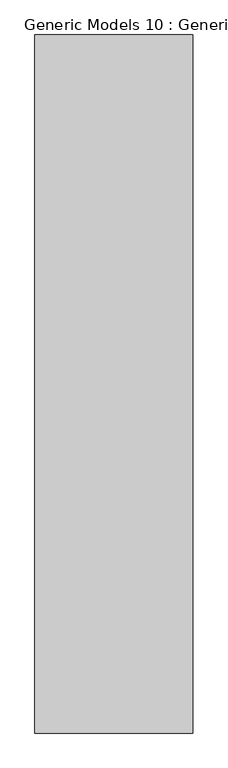
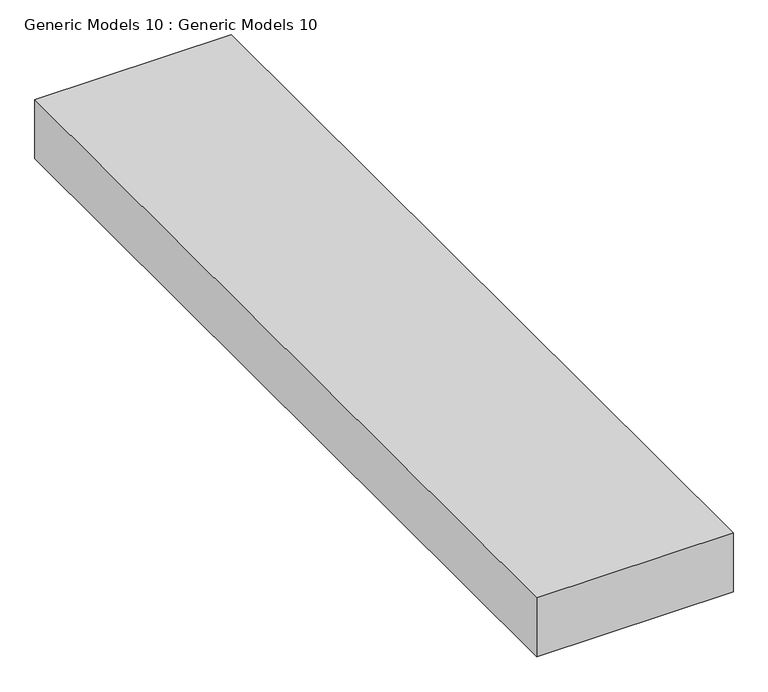
"""IFC4 building model written with IfcOpenShell, lengths in millimetres: proxy geometry, Generic Models 10 : Generic Models 10."""

from ifc_helpers import new_model, si_unit, frame, origin, place, context, project, spatial, polyline, outline, extrude, source, transform, mapped, element, save


def generic_models_10_generic_models_10_e59920a7(model_context):
    return source(origin(), model_context, "Body", "SweptSolid", [
        extrude(outline(polyline([(-3320.2262478, 2441.9722768), (-3320.2262478, 307.998934), (-3802.4859258, 307.998934), (-3802.4859258, 2441.9722768), (-3320.2262478, 2441.9722768)])), frame((0.0, 0.0, 5279.0460342), z_axis=(0.0, 0.0, 1.0), x_axis=(1.0, 0.0, 0.0)), (0.0, 0.0, 1.0), 152.4),
    ])


if __name__ == "__main__":
    model = new_model("IFC4")
    model_context = context("Model", 3, world=origin())
    ifc_project = project(units=[si_unit("LENGTHUNIT", "METRE", prefix="MILLI")], contexts=[model_context])
    site = spatial("IfcSite", under=ifc_project)
    building = spatial("IfcBuilding", under=site)
    placement = place(None, origin())
    generic_models_10_generic_models_10_shape = generic_models_10_generic_models_10_e59920a7(model_context)
    element("IfcBuildingElementProxy", 1, Name="Generic Models 10 : Generic Models 10", ObjectType="Generic Models 10 : Generic Models 10", at=placement, inside=building, context=model_context, shape_type="MappedRepresentation", body=[
        mapped(generic_models_10_generic_models_10_shape, transform((0.0, 0.0, 0.0), x_axis=(1.0, 0.0, 0.0), y_axis=(0.0, 1.0, 0.0), z_axis=(0.0, 0.0, 1.0))),
    ])
    save(model, "model.ifc")
